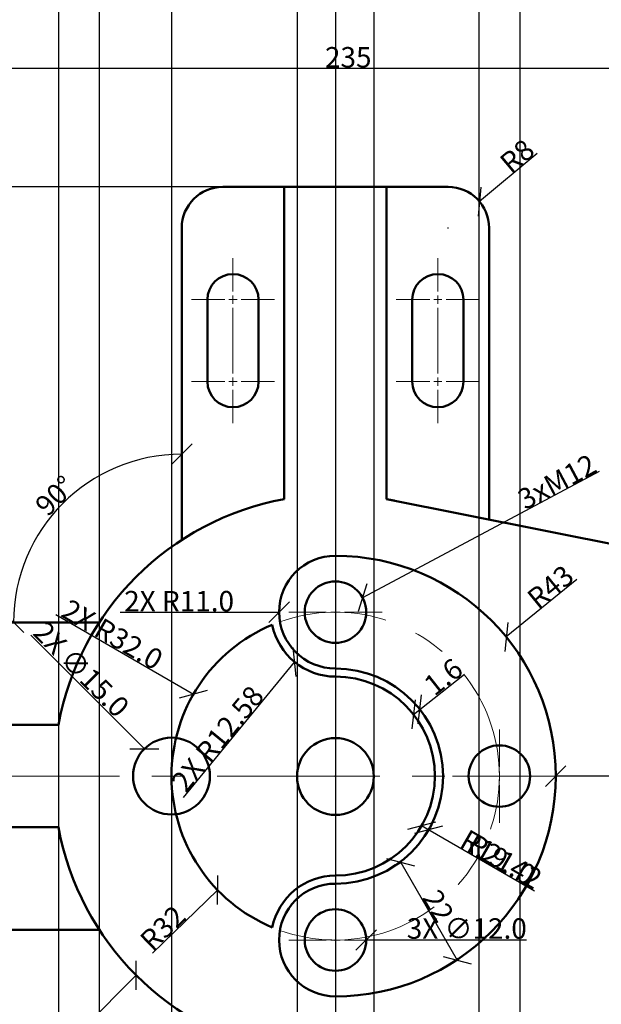
# Model space of a CAD drawing. Units: millimetres. Extents: x 263 to 611, y 50 to 522.
# Tile 3 of 5: x 364 to 478, y 157 to 349. Entities that reach past the tile are written whole.
import ezdxf

# ---------------------------------------------------------------- set-up
doc = ezdxf.new("R2010")
doc.units = ezdxf.units.MM
doc.header["$MEASUREMENT"] = 0
doc.linetypes.add('CENTER', pattern=[50.8, 31.75, -6.35, 6.35, -6.35])
for name, color, linetype, lineweight in [('M-CNTR', 1, 'CENTER', 18), ('M-DIMS', 2, 'Continuous', 25), ('M-OUTL', 7, 'Continuous', 50)]:
    doc.layers.add(name, color=color, linetype=linetype, lineweight=lineweight)
doc.styles.get("Standard").update_dxf_attribs({"font": 'arial.ttf'})
doc.dimstyles.get("Standard").update_dxf_attribs({"dimtxt": 4, "dimasz": 4, "dimexe": 0.18, "dimexo": 0.0625, "dimgap": 0.09, "dimtad": 1, "dimdec": 0, "dimzin": 0, "dimdsep": 46, "dimtxsty": 'Standard', "dimblk": 'OBLIQUE', "dimcen": 0.09, "dimclre": 251, "dimadec": 0, "dimazin": 0, "dimtfac": 1, "dimtdec": 0, "dimtofl": 0, "dimtmove": 0, "dimatfit": 3, "dimfxl": 1, "dimtolj": 1, "dimtzin": 0, "dimarcsym": 0})

# ---------------------------------------------------------------- blocks, each defined once
blk = doc.blocks.new('*U2')
at = {"layer": 'M-CNTR', "color": 0, "transparency": 16777216}
for p, q in [((0, 1.8), (0, 9.12)), ((-9.12, 0), (-1.8, 0)), ((1.8, 0), (9.12, 0)), ((0, -9.12), (0, -1.8))]:
    blk.add_line(p, q, dxfattribs=at)
at = {"layer": 'M-CNTR', "color": 0, "linetype": 'Continuous', "transparency": 16777216}
for p, q in [((-0.9, 0), (0.9, 0)), ((0, -0.9), (0, 0.9))]:
    blk.add_line(p, q, dxfattribs=at)
blk = doc.blocks.new('*U3')
at = {"layer": 'M-CNTR', "color": 0, "transparency": 16777216}
for p, q in [((0, 1.8), (0, 9.12)), ((-9.12, 0), (-1.8, 0)), ((1.8, 0), (9.12, 0)), ((0, -9.12), (0, -1.8))]:
    blk.add_line(p, q, dxfattribs=at)
at = {"layer": 'M-CNTR', "color": 0, "linetype": 'Continuous', "transparency": 16777216}
for p, q in [((-0.9, 0), (0.9, 0)), ((0, -0.9), (0, 0.9))]:
    blk.add_line(p, q, dxfattribs=at)
blk = doc.blocks.new('*U4')
at = {"layer": 'M-CNTR', "color": 0, "transparency": 16777216}
for p, q in [((0, 1.8), (0, 9.12)), ((-9.12, 0), (-1.8, 0)), ((1.8, 0), (9.12, 0)), ((0, -9.12), (0, -1.8))]:
    blk.add_line(p, q, dxfattribs=at)
at = {"layer": 'M-CNTR', "color": 0, "linetype": 'Continuous', "transparency": 16777216}
for p, q in [((-0.9, 0), (0.9, 0)), ((0, -0.9), (0, 0.9))]:
    blk.add_line(p, q, dxfattribs=at)
blk = doc.blocks.new('*U14')
at = {"layer": 'M-CNTR', "color": 0, "transparency": 16777216}
for p, q in [((0, 1.6), (0, 8.12)), ((-8.12, 0), (-1.6, 0)), ((1.6, 0), (8.12, 0)), ((0, -8.12), (0, -1.6))]:
    blk.add_line(p, q, dxfattribs=at)
at = {"layer": 'M-CNTR', "color": 0, "linetype": 'Continuous', "transparency": 16777216}
for p, q in [((-0.8, 0), (0.8, 0)), ((0, -0.8), (0, 0.8))]:
    blk.add_line(p, q, dxfattribs=at)
blk = doc.blocks.new('*U15')
at = {"layer": 'M-CNTR', "color": 0, "transparency": 16777216}
for p, q in [((0, 1.6), (0, 8.12)), ((-8.12, 0), (-1.6, 0)), ((1.6, 0), (8.12, 0)), ((0, -8.12), (0, -1.6))]:
    blk.add_line(p, q, dxfattribs=at)
at = {"layer": 'M-CNTR', "color": 0, "linetype": 'Continuous', "transparency": 16777216}
for p, q in [((-0.8, 0), (0.8, 0)), ((0, -0.8), (0, 0.8))]:
    blk.add_line(p, q, dxfattribs=at)
blk = doc.blocks.new('*U16')
at = {"layer": 'M-CNTR', "color": 0, "transparency": 16777216}
for p, q in [((0, 1.6), (0, 8.12)), ((-8.12, 0), (-1.6, 0)), ((1.6, 0), (8.12, 0)), ((0, -8.12), (0, -1.6))]:
    blk.add_line(p, q, dxfattribs=at)
at = {"layer": 'M-CNTR', "color": 0, "linetype": 'Continuous', "transparency": 16777216}
for p, q in [((-0.8, 0), (0.8, 0)), ((0, -0.8), (0, 0.8))]:
    blk.add_line(p, q, dxfattribs=at)
blk = doc.blocks.new('*U17')
at = {"layer": 'M-CNTR', "color": 0, "transparency": 16777216}
for p, q in [((0, 1.6), (0, 8.12)), ((-8.12, 0), (-1.6, 0)), ((1.6, 0), (8.12, 0)), ((0, -8.12), (0, -1.6))]:
    blk.add_line(p, q, dxfattribs=at)
at = {"layer": 'M-CNTR', "color": 0, "linetype": 'Continuous', "transparency": 16777216}
for p, q in [((-0.8, 0), (0.8, 0)), ((0, -0.8), (0, 0.8))]:
    blk.add_line(p, q, dxfattribs=at)
blk = doc.blocks.new('_Oblique')
at = {"color": 0, "linetype": 'ByBlock', "lineweight": -2}
blk.add_line((-0.5, -0.5), (0.5, 0.5), dxfattribs=at)
blk = doc.blocks.new('*D18')
at = {"layer": 'Defpoints', "color": 0, "transparency": 16777216}
for p in [(546.1, 339.25), (546.1, 231.08), (311.1, 223.08)]:
    blk.add_point(p, dxfattribs=at)
at = {"layer": 'M-DIMS', "color": 0, "lineweight": -2, "transparency": 16777216}
for p, q in [((311.1, 223.14), (311.1, 339.43)), ((311.1, 339.25), (546.1, 339.25)), ((546.1, 231.14), (546.1, 339.43))]:
    blk.add_line(p, q, dxfattribs=at)
at = {"layer": 'M-DIMS', "color": 0, "lineweight": -2, "transparency": 16777216, "xscale": 4, "yscale": 4, "zscale": 4, "rotation": 180}
blk.add_blockref('_Oblique', (311.1, 339.25), dxfattribs=at)
at = {"layer": 'M-DIMS', "color": 0, "lineweight": -2, "transparency": 16777216, "xscale": 4, "yscale": 4, "zscale": 4}
blk.add_blockref('_Oblique', (546.1, 339.25), dxfattribs=at)
at = {"layer": 'M-DIMS', "color": 0, "transparency": 16777216, "insert": (428.6, 341.39), "char_height": 4, "attachment_point": 5}
blk.add_mtext('\\A1;235', dxfattribs=at)
blk = doc.blocks.new('*D21')
at = {"layer": 'Defpoints', "color": 0, "transparency": 16777216}
for p in [(282.64, 316.08), (404.1, 316.08), (319.1, 231.08)]:
    blk.add_point(p, dxfattribs=at)
at = {"layer": 'M-DIMS', "color": 0, "lineweight": -2, "transparency": 16777216}
for p, q in [((404.04, 316.08), (282.46, 316.08)), ((282.64, 231.08), (282.64, 316.08)), ((319.04, 231.08), (282.46, 231.08))]:
    blk.add_line(p, q, dxfattribs=at)
at = {"layer": 'M-DIMS', "color": 0, "lineweight": -2, "transparency": 16777216, "xscale": 4, "yscale": 4, "zscale": 4}
for p, rotation in [((282.64, 316.08), 90), ((282.64, 231.08), 270)]:
    blk.add_blockref('_Oblique', p, dxfattribs=dict(at, rotation=rotation))
at = {"layer": 'M-DIMS', "color": 0, "transparency": 16777216, "insert": (280.51, 273.58), "char_height": 4, "attachment_point": 5, "rotation": 90}
blk.add_mtext('\\A1;85', dxfattribs=at)
blk = doc.blocks.new('*D22')
at = {"layer": 'Defpoints', "color": 0, "transparency": 16777216}
for p in [(404.1, 316.08), (267.8, 86.08), (404.1, 86.08)]:
    blk.add_point(p, dxfattribs=at)
at = {"layer": 'M-DIMS', "color": 0, "lineweight": -2, "transparency": 16777216}
for p, q in [((404.04, 316.08), (267.62, 316.08)), ((267.8, 316.08), (267.8, 86.08)), ((404.04, 86.08), (267.62, 86.08))]:
    blk.add_line(p, q, dxfattribs=at)
at = {"layer": 'M-DIMS', "color": 0, "lineweight": -2, "transparency": 16777216, "xscale": 4, "yscale": 4, "zscale": 4}
for p, rotation in [((267.8, 316.08), 90), ((267.8, 86.08), 270)]:
    blk.add_blockref('_Oblique', p, dxfattribs=dict(at, rotation=rotation))
at = {"layer": 'M-DIMS', "color": 0, "transparency": 16777216, "insert": (265.67, 201.08), "char_height": 4, "attachment_point": 5, "rotation": 90}
blk.add_mtext('\\A1;230', dxfattribs=at)
blk = doc.blocks.new('*D25')
at = {"layer": 'Defpoints', "color": 0, "transparency": 16777216}
for p in [(311.1, 201.08), (426.1, 201.08), (426.1, 140.57)]:
    blk.add_point(p, dxfattribs=at)
at = {"layer": 'M-DIMS', "color": 0, "lineweight": -2, "transparency": 16777216}
for p, q in [((311.1, 201.02), (311.1, 140.39)), ((426.1, 201.02), (426.1, 140.39)), ((311.1, 140.57), (426.1, 140.57))]:
    blk.add_line(p, q, dxfattribs=at)
at = {"layer": 'M-DIMS', "color": 0, "lineweight": -2, "transparency": 16777216, "xscale": 4, "yscale": 4, "zscale": 4, "rotation": 180}
blk.add_blockref('_Oblique', (311.1, 140.57), dxfattribs=at)
at = {"layer": 'M-DIMS', "color": 0, "lineweight": -2, "transparency": 16777216, "xscale": 4, "yscale": 4, "zscale": 4}
blk.add_blockref('_Oblique', (426.1, 140.57), dxfattribs=at)
at = {"layer": 'M-DIMS', "color": 0, "transparency": 16777216, "insert": (368.6, 142.7), "char_height": 4, "attachment_point": 5}
blk.add_mtext('\\A1;115', dxfattribs=at)
blk = doc.blocks.new('*D26')
at = {"layer": 'Defpoints', "color": 0, "transparency": 16777216}
for p in [(436.59, 182.89), (447.58, 163.83), (449.87, 165.15)]:
    blk.add_point(p, dxfattribs=at)
at = {"layer": 'M-DIMS', "color": 0, "lineweight": -2, "transparency": 16777216}
for p, q in [((436.64, 182.92), (439.04, 184.3)), ((438.88, 184.21), (449.87, 165.15)), ((447.64, 163.86), (450.03, 165.24))]:
    blk.add_line(p, q, dxfattribs=at)
at = {"layer": 'M-DIMS', "color": 0, "lineweight": -2, "transparency": 16777216, "xscale": 4, "yscale": 4, "zscale": 4}
for p, rotation in [((438.88, 184.21), 119.9728507659306), ((449.87, 165.15), 299.9728507659306)]:
    blk.add_blockref('_Oblique', p, dxfattribs=dict(at, rotation=rotation))
at = {"layer": 'M-DIMS', "color": 0, "transparency": 16777216, "insert": (446.19, 175.73), "char_height": 4, "attachment_point": 5, "rotation": 299.9729}
blk.add_mtext('\\A1;22', dxfattribs=at)
blk = doc.blocks.new('*D29')
at = {"layer": 'Defpoints', "color": 0, "transparency": 16777216}
for p in [(396.1, 308.08), (379.68, 259.52), (396.1, 247.18), (319.1, 231.08), (380, 231.08)]:
    blk.add_point(p, dxfattribs=at)
at = {"layer": 'M-DIMS', "color": 0, "lineweight": -2, "transparency": 16777216}
blk.add_arc((396.1, 231.08), 32.84, 90, 180, dxfattribs=at)
at = {"layer": 'M-DIMS', "color": 0, "lineweight": -2, "transparency": 16777216, "xscale": 4, "yscale": 4, "zscale": 4}
for p, rotation in [((396.1, 263.92), 359.9999999999999), ((363.26, 231.08), 269.9999999999999)]:
    blk.add_blockref('_Oblique', p, dxfattribs=dict(at, rotation=rotation))
at = {"layer": 'M-DIMS', "color": 0, "transparency": 16777216, "insert": (371.37, 255.81), "char_height": 4, "attachment_point": 5, "rotation": 45}
blk.add_mtext('\\A1;90°', dxfattribs=at)
blk = doc.blocks.new('*D30')
at = {"layer": 'Defpoints', "color": 0, "transparency": 16777216}
for p in [(454.24, 313.21), (448.1, 308.08)]:
    blk.add_point(p, dxfattribs=at)
at = {"layer": 'M-DIMS', "color": 0, "lineweight": -2, "transparency": 16777216}
for p, q in [((465.48, 322.59), (454.24, 313.21)), ((448.01, 308.08), (448.19, 308.08)), ((448.1, 307.99), (448.1, 308.17))]:
    blk.add_line(p, q, dxfattribs=at)
at = {"layer": 'M-DIMS', "color": 0, "lineweight": -2, "transparency": 16777216, "xscale": 4, "yscale": 4, "zscale": 4, "rotation": 219.8589270898177}
blk.add_blockref('_Oblique', (454.24, 313.21), dxfattribs=at)
at = {"layer": 'M-DIMS', "color": 0, "transparency": 16777216, "insert": (461.56, 322.1), "char_height": 4, "attachment_point": 5, "rotation": 39.8589}
blk.add_mtext('\\A1;R8', dxfattribs=at)
blk = doc.blocks.new('*D31')
at = {"layer": 'Defpoints', "color": 0, "transparency": 16777216}
for p in [(459.44, 228.24), (426.1, 201.08)]:
    blk.add_point(p, dxfattribs=at)
at = {"layer": 'M-DIMS', "color": 0, "lineweight": -2, "transparency": 16777216}
for p, q in [((473.19, 239.44), (459.44, 228.24)), ((426.01, 201.08), (426.19, 201.08)), ((426.1, 200.99), (426.1, 201.17))]:
    blk.add_line(p, q, dxfattribs=at)
at = {"layer": 'M-DIMS', "color": 0, "lineweight": -2, "transparency": 16777216, "xscale": 4, "yscale": 4, "zscale": 4, "rotation": 219.1694218645044}
blk.add_blockref('_Oblique', (459.44, 228.24), dxfattribs=at)
at = {"layer": 'M-DIMS', "color": 0, "transparency": 16777216, "insert": (468.07, 238.02), "char_height": 4, "attachment_point": 5, "rotation": 39.1694}
blk.add_mtext('\\A1;R43', dxfattribs=at)
blk = doc.blocks.new('*D32')
at = {"layer": 'Defpoints', "color": 0, "transparency": 16777216}
for p in [(426.1, 201.08), (403.1, 178.83)]:
    blk.add_point(p, dxfattribs=at)
at = {"layer": 'M-DIMS', "color": 0, "lineweight": -2, "transparency": 16777216}
for p, q in [((426.01, 201.08), (426.19, 201.08)), ((426.1, 200.99), (426.1, 201.17)), ((390.38, 166.52), (403.1, 178.83))]:
    blk.add_line(p, q, dxfattribs=at)
at = {"layer": 'M-DIMS', "color": 0, "lineweight": -2, "transparency": 16777216, "xscale": 4, "yscale": 4, "zscale": 4, "rotation": 44.055010952388}
blk.add_blockref('_Oblique', (403.1, 178.83), dxfattribs=at)
at = {"layer": 'M-DIMS', "color": 0, "transparency": 16777216, "insert": (392.38, 171.43), "char_height": 4, "attachment_point": 5, "rotation": 44.055}
blk.add_mtext('\\A1;R32', dxfattribs=at)
blk = doc.blocks.new('*D33')
at = {"layer": 'Defpoints', "color": 0, "transparency": 16777216}
for p in [(442.57, 214.11), (442.57, 214.11), (441.33, 213.13)]:
    blk.add_point(p, dxfattribs=at)
at = {"layer": 'M-DIMS', "color": 0, "lineweight": -2, "transparency": 16777216}
for p, q in [((442.57, 214.11), (451.26, 220.98)), ((441.33, 213.13), (442.57, 214.11)), ((442.61, 214.06), (442.68, 213.97)), ((441.37, 213.08), (441.44, 212.99))]:
    blk.add_line(p, q, dxfattribs=at)
at = {"layer": 'M-DIMS', "color": 0, "lineweight": -2, "transparency": 16777216, "xscale": 4, "yscale": 4, "zscale": 4}
for p, rotation in [((441.33, 213.13), 218.3421878076332), ((442.57, 214.11), 38.34218780763318)]:
    blk.add_blockref('_Oblique', p, dxfattribs=dict(at, rotation=rotation))
at = {"layer": 'M-DIMS', "color": 0, "transparency": 16777216, "insert": (447.16, 220.46), "char_height": 4, "attachment_point": 5, "rotation": 38.3422}
blk.add_mtext('\\A1;1.6', dxfattribs=at)
blk = doc.blocks.new('*D35')
at = {"layer": 'Defpoints', "color": 0, "transparency": 16777216}
for p in [(431.39, 235.9), (420.8, 230.26)]:
    blk.add_point(p, dxfattribs=at)
at = {"layer": 'M-DIMS', "color": 0, "lineweight": -2, "transparency": 16777216}
for p, q in [((477.59, 260.53), (431.39, 235.9)), ((426.01, 233.08), (426.19, 233.08)), ((426.1, 232.99), (426.1, 233.17))]:
    blk.add_line(p, q, dxfattribs=at)
at = {"layer": 'M-DIMS', "color": 0, "lineweight": -2, "transparency": 16777216, "xscale": 4, "yscale": 4, "zscale": 4, "rotation": 208.0625642859589}
blk.add_blockref('_Oblique', (431.39, 235.9), dxfattribs=at)
at = {"layer": 'M-DIMS', "color": 0, "transparency": 16777216, "insert": (469.34, 258.55), "char_height": 4, "attachment_point": 5, "rotation": 28.0626}
blk.add_mtext('\\A1;3xM12', dxfattribs=at)
blk = doc.blocks.new('SLOT-10x26')
for p, q in [((0, 5), (0, 21)), ((10, 5), (10, 21))]:
    blk.add_line(p, q)
for centre, start, end in [((5, 21), 0, 180), ((5, 5), 180, 0)]:
    blk.add_arc(centre, 5, start, end)
blk = doc.blocks.new('*D53')
at = {"layer": 'Defpoints', "color": 0, "transparency": 16777216}
for p in [(578.1, 423.27), (311.1, 383.27), (578.1, 52.26)]:
    blk.add_point(p, dxfattribs=at)
at = {"layer": 'M-DIMS', "color": 251, "lineweight": -2, "transparency": 16777216}
for p, q in [((578.1, 423.21), (578.1, 52.08)), ((311.1, 383.21), (311.1, 52.08))]:
    blk.add_line(p, q, dxfattribs=at)
at = {"layer": 'M-DIMS', "color": 0, "lineweight": -2, "transparency": 16777216}
blk.add_line((311.1, 52.26), (578.1, 52.26), dxfattribs=at)
at = {"layer": 'M-DIMS', "color": 0, "lineweight": -2, "transparency": 16777216, "xscale": 4, "yscale": 4, "zscale": 4, "rotation": 180}
blk.add_blockref('_Oblique', (311.1, 52.26), dxfattribs=at)
at = {"layer": 'M-DIMS', "color": 0, "lineweight": -2, "transparency": 16777216, "xscale": 4, "yscale": 4, "zscale": 4}
blk.add_blockref('_Oblique', (578.1, 52.26), dxfattribs=at)
at = {"layer": 'M-DIMS', "color": 0, "transparency": 16777216, "insert": (444.6, 54.39), "char_height": 4, "attachment_point": 5}
blk.add_mtext('\\A1;267.0', dxfattribs=at)
blk = doc.blocks.new('*D56')
at = {"layer": 'Defpoints', "color": 0, "transparency": 16777216}
for p in [(454.1, 410.27), (462.1, 410.27), (462.1, 52.26)]:
    blk.add_point(p, dxfattribs=at)
at = {"layer": 'M-DIMS', "color": 251, "lineweight": -2, "transparency": 16777216}
for p, q in [((454.1, 410.21), (454.1, 52.08)), ((462.1, 410.21), (462.1, 52.08))]:
    blk.add_line(p, q, dxfattribs=at)
at = {"layer": 'M-DIMS', "color": 0, "lineweight": -2, "transparency": 16777216}
blk.add_line((454.1, 52.26), (462.1, 52.26), dxfattribs=at)
at = {"layer": 'M-DIMS', "color": 0, "lineweight": -2, "transparency": 16777216, "xscale": 4, "yscale": 4, "zscale": 4, "rotation": 180}
blk.add_blockref('_Oblique', (454.1, 52.26), dxfattribs=at)
at = {"layer": 'M-DIMS', "color": 0, "lineweight": -2, "transparency": 16777216, "xscale": 4, "yscale": 4, "zscale": 4}
blk.add_blockref('_Oblique', (462.1, 52.26), dxfattribs=at)
at = {"layer": 'M-DIMS', "color": 0, "transparency": 16777216, "insert": (458.1, 54.39), "char_height": 4, "attachment_point": 5}
blk.add_mtext('\\A1;8.0', dxfattribs=at)
blk = doc.blocks.new('*D57')
at = {"layer": 'Defpoints', "color": 0, "transparency": 16777216}
for p in [(372.02, 403.27), (311.1, 383.27), (372.02, 52.26)]:
    blk.add_point(p, dxfattribs=at)
at = {"layer": 'M-DIMS', "color": 251, "lineweight": -2, "transparency": 16777216}
for p, q in [((372.02, 403.21), (372.02, 52.08)), ((311.1, 383.21), (311.1, 52.08))]:
    blk.add_line(p, q, dxfattribs=at)
at = {"layer": 'M-DIMS', "color": 0, "lineweight": -2, "transparency": 16777216}
blk.add_line((311.1, 52.26), (372.02, 52.26), dxfattribs=at)
at = {"layer": 'M-DIMS', "color": 0, "lineweight": -2, "transparency": 16777216, "xscale": 4, "yscale": 4, "zscale": 4, "rotation": 180}
blk.add_blockref('_Oblique', (311.1, 52.26), dxfattribs=at)
at = {"layer": 'M-DIMS', "color": 0, "lineweight": -2, "transparency": 16777216, "xscale": 4, "yscale": 4, "zscale": 4}
blk.add_blockref('_Oblique', (372.02, 52.26), dxfattribs=at)
at = {"layer": 'M-DIMS', "color": 0, "transparency": 16777216, "insert": (341.56, 54.39), "char_height": 4, "attachment_point": 5}
blk.add_mtext('\\A1;60.92', dxfattribs=at)
blk = doc.blocks.new('*D58')
at = {"layer": 'Defpoints', "color": 0, "transparency": 16777216}
for p in [(372.02, 403.27), (380, 383.27), (380, 52.26)]:
    blk.add_point(p, dxfattribs=at)
at = {"layer": 'M-DIMS', "color": 251, "lineweight": -2, "transparency": 16777216}
for p, q in [((372.02, 403.21), (372.02, 52.08)), ((380, 383.21), (380, 52.08))]:
    blk.add_line(p, q, dxfattribs=at)
at = {"layer": 'M-DIMS', "color": 0, "lineweight": -2, "transparency": 16777216}
for p, q in [((372.02, 52.26), (380, 52.26)), ((380, 52.26), (397.64, 52.26))]:
    blk.add_line(p, q, dxfattribs=at)
at = {"layer": 'M-DIMS', "color": 0, "lineweight": -2, "transparency": 16777216, "xscale": 4, "yscale": 4, "zscale": 4, "rotation": 180}
blk.add_blockref('_Oblique', (372.02, 52.26), dxfattribs=at)
at = {"layer": 'M-DIMS', "color": 0, "lineweight": -2, "transparency": 16777216, "xscale": 4, "yscale": 4, "zscale": 4}
blk.add_blockref('_Oblique', (380, 52.26), dxfattribs=at)
at = {"layer": 'M-DIMS', "color": 0, "transparency": 16777216, "insert": (390.82, 54.39), "char_height": 4, "attachment_point": 5}
blk.add_mtext('\\A1;7.986', dxfattribs=at)
blk = doc.blocks.new('*D59')
at = {"layer": 'Defpoints', "color": 0, "transparency": 16777216}
for p in [(380, 383.27), (394.1, 383.27), (394.1, 52.26)]:
    blk.add_point(p, dxfattribs=at)
at = {"layer": 'M-DIMS', "color": 251, "lineweight": -2, "transparency": 16777216}
for p, q in [((380, 383.21), (380, 52.08)), ((394.1, 383.21), (394.1, 52.08))]:
    blk.add_line(p, q, dxfattribs=at)
at = {"layer": 'M-DIMS', "color": 0, "lineweight": -2, "transparency": 16777216}
for p, q in [((380, 52.26), (394.1, 52.26)), ((394.1, 52.26), (414.52, 52.26))]:
    blk.add_line(p, q, dxfattribs=at)
at = {"layer": 'M-DIMS', "color": 0, "lineweight": -2, "transparency": 16777216, "xscale": 4, "yscale": 4, "zscale": 4, "rotation": 180}
blk.add_blockref('_Oblique', (380, 52.26), dxfattribs=at)
at = {"layer": 'M-DIMS', "color": 0, "lineweight": -2, "transparency": 16777216, "xscale": 4, "yscale": 4, "zscale": 4}
blk.add_blockref('_Oblique', (394.1, 52.26), dxfattribs=at)
at = {"layer": 'M-DIMS', "color": 0, "transparency": 16777216, "insert": (406.31, 54.39), "char_height": 4, "attachment_point": 5}
blk.add_mtext('\\A1;14.098', dxfattribs=at)
blk = doc.blocks.new('*D60')
at = {"layer": 'Defpoints', "color": 0, "transparency": 16777216}
for p in [(418.6, 403.27), (394.1, 383.27), (418.6, 52.26)]:
    blk.add_point(p, dxfattribs=at)
at = {"layer": 'M-DIMS', "color": 251, "lineweight": -2, "transparency": 16777216}
for p, q in [((418.6, 403.21), (418.6, 52.08)), ((394.1, 383.21), (394.1, 52.08))]:
    blk.add_line(p, q, dxfattribs=at)
at = {"layer": 'M-DIMS', "color": 0, "lineweight": -2, "transparency": 16777216}
blk.add_line((394.1, 52.26), (418.6, 52.26), dxfattribs=at)
at = {"layer": 'M-DIMS', "color": 0, "lineweight": -2, "transparency": 16777216, "xscale": 4, "yscale": 4, "zscale": 4, "rotation": 180}
blk.add_blockref('_Oblique', (394.1, 52.26), dxfattribs=at)
at = {"layer": 'M-DIMS', "color": 0, "lineweight": -2, "transparency": 16777216, "xscale": 4, "yscale": 4, "zscale": 4}
blk.add_blockref('_Oblique', (418.6, 52.26), dxfattribs=at)
at = {"layer": 'M-DIMS', "color": 0, "transparency": 16777216, "insert": (406.35, 54.39), "char_height": 4, "attachment_point": 5}
blk.add_mtext('\\A1;24.5', dxfattribs=at)
blk = doc.blocks.new('*D61')
at = {"layer": 'Defpoints', "color": 0, "transparency": 16777216}
for p in [(418.6, 403.27), (426.1, 378.63), (426.1, 52.26)]:
    blk.add_point(p, dxfattribs=at)
at = {"layer": 'M-DIMS', "color": 251, "lineweight": -2, "transparency": 16777216}
for p, q in [((418.6, 403.21), (418.6, 52.08)), ((426.1, 378.57), (426.1, 52.08))]:
    blk.add_line(p, q, dxfattribs=at)
at = {"layer": 'M-DIMS', "color": 0, "lineweight": -2, "transparency": 16777216}
blk.add_line((418.6, 52.26), (426.1, 52.26), dxfattribs=at)
at = {"layer": 'M-DIMS', "color": 0, "lineweight": -2, "transparency": 16777216, "xscale": 4, "yscale": 4, "zscale": 4, "rotation": 180}
blk.add_blockref('_Oblique', (418.6, 52.26), dxfattribs=at)
at = {"layer": 'M-DIMS', "color": 0, "lineweight": -2, "transparency": 16777216, "xscale": 4, "yscale": 4, "zscale": 4}
blk.add_blockref('_Oblique', (426.1, 52.26), dxfattribs=at)
at = {"layer": 'M-DIMS', "color": 0, "transparency": 16777216, "insert": (422.35, 54.38), "char_height": 4, "attachment_point": 5}
blk.add_mtext('\\A1;7.5', dxfattribs=at)
blk = doc.blocks.new('*D62')
at = {"layer": 'Defpoints', "color": 0, "transparency": 16777216}
for p in [(433.6, 383.27), (426.1, 378.63), (433.6, 52.26)]:
    blk.add_point(p, dxfattribs=at)
at = {"layer": 'M-DIMS', "color": 251, "lineweight": -2, "transparency": 16777216}
for p, q in [((433.6, 383.21), (433.6, 52.08)), ((426.1, 378.57), (426.1, 52.08))]:
    blk.add_line(p, q, dxfattribs=at)
at = {"layer": 'M-DIMS', "color": 0, "lineweight": -2, "transparency": 16777216}
blk.add_line((426.1, 52.26), (433.6, 52.26), dxfattribs=at)
at = {"layer": 'M-DIMS', "color": 0, "lineweight": -2, "transparency": 16777216, "xscale": 4, "yscale": 4, "zscale": 4, "rotation": 180}
blk.add_blockref('_Oblique', (426.1, 52.26), dxfattribs=at)
at = {"layer": 'M-DIMS', "color": 0, "lineweight": -2, "transparency": 16777216, "xscale": 4, "yscale": 4, "zscale": 4}
blk.add_blockref('_Oblique', (433.6, 52.26), dxfattribs=at)
at = {"layer": 'M-DIMS', "color": 0, "transparency": 16777216, "insert": (429.85, 54.38), "char_height": 4, "attachment_point": 5}
blk.add_mtext('\\A1;7.5', dxfattribs=at)
blk = doc.blocks.new('*D69')
at = {"layer": 'Defpoints', "color": 0, "transparency": 16777216}
for p in [(426.1, 201.08), (387.21, 162.19)]:
    blk.add_point(p, dxfattribs=at)
at = {"layer": 'M-DIMS', "color": 251, "lineweight": -2, "transparency": 16777216}
for p, q in [((426.01, 201.08), (426.19, 201.08)), ((426.1, 200.99), (426.1, 201.17))]:
    blk.add_line(p, q, dxfattribs=at)
at = {"layer": 'M-DIMS', "color": 0, "lineweight": -2, "transparency": 16777216}
blk.add_line((355.69, 130.68), (387.21, 162.19), dxfattribs=at)
at = {"layer": 'M-DIMS', "color": 0, "lineweight": -2, "transparency": 16777216, "xscale": 4, "yscale": 4, "zscale": 4, "rotation": 44.99977533015295}
blk.add_blockref('_Oblique', (387.21, 162.19), dxfattribs=at)
at = {"layer": 'M-DIMS', "color": 0, "transparency": 16777216, "insert": (362.37, 140.36), "char_height": 4, "attachment_point": 5, "rotation": 44.9998}
blk.add_mtext('\\A1;4X R55.0', dxfattribs=at)
blk = doc.blocks.new('*D70')
at = {"layer": 'Defpoints', "color": 0, "transparency": 16777216}
for p in [(426.1, 201.08), (469.1, 201.08)]:
    blk.add_point(p, dxfattribs=at)
at = {"layer": 'M-DIMS', "color": 251, "lineweight": -2, "transparency": 16777216}
for p, q in [((426.01, 201.08), (426.19, 201.08)), ((426.1, 200.99), (426.1, 201.17))]:
    blk.add_line(p, q, dxfattribs=at)
at = {"layer": 'M-DIMS', "color": 0, "lineweight": -2, "transparency": 16777216}
blk.add_line((502.09, 201.08), (469.1, 201.08), dxfattribs=at)
at = {"layer": 'M-DIMS', "color": 0, "lineweight": -2, "transparency": 16777216, "xscale": 4, "yscale": 4, "zscale": 4, "rotation": 180.0006262561947}
blk.add_blockref('_Oblique', (469.1, 201.08), dxfattribs=at)
at = {"layer": 'M-DIMS', "color": 0, "transparency": 16777216, "insert": (494.9, 203.22), "char_height": 4, "attachment_point": 5, "rotation": 0.0006}
blk.add_mtext('\\A1;R43.0', dxfattribs=at)
blk = doc.blocks.new('*D71')
at = {"layer": 'Defpoints', "color": 0, "transparency": 16777216}
for p in [(398.4, 217.1), (426.1, 201.08)]:
    blk.add_point(p, dxfattribs=at)
at = {"layer": 'M-DIMS', "color": 0, "lineweight": -2, "transparency": 16777216}
blk.add_line((371.52, 232.64), (398.4, 217.1), dxfattribs=at)
at = {"layer": 'M-DIMS', "color": 251, "lineweight": -2, "transparency": 16777216}
for p, q in [((426.01, 201.08), (426.19, 201.08)), ((426.1, 200.99), (426.1, 201.17))]:
    blk.add_line(p, q, dxfattribs=at)
at = {"layer": 'M-DIMS', "color": 0, "lineweight": -2, "transparency": 16777216, "xscale": 4, "yscale": 4, "zscale": 4, "rotation": 329.9588428914435}
blk.add_blockref('_Oblique', (398.4, 217.1), dxfattribs=at)
at = {"layer": 'M-DIMS', "color": 0, "transparency": 16777216, "insert": (382.56, 228.72), "char_height": 4, "attachment_point": 5, "rotation": 329.9588}
blk.add_mtext('\\A1;2X R32.0', dxfattribs=at)
blk = doc.blocks.new('*D74')
at = {"layer": 'Defpoints', "color": 0, "transparency": 16777216}
for p in [(426.1, 201.08), (442.92, 191.37)]:
    blk.add_point(p, dxfattribs=at)
at = {"layer": 'M-DIMS', "color": 251, "lineweight": -2, "transparency": 16777216}
for p, q in [((426.01, 201.08), (426.19, 201.08)), ((426.1, 200.99), (426.1, 201.17))]:
    blk.add_line(p, q, dxfattribs=at)
at = {"layer": 'M-DIMS', "color": 0, "lineweight": -2, "transparency": 16777216}
blk.add_line((464.97, 178.64), (442.92, 191.37), dxfattribs=at)
at = {"layer": 'M-DIMS', "color": 0, "lineweight": -2, "transparency": 16777216, "xscale": 4, "yscale": 4, "zscale": 4, "rotation": 150.0004448494699}
blk.add_blockref('_Oblique', (442.92, 191.37), dxfattribs=at)
at = {"layer": 'M-DIMS', "color": 0, "transparency": 16777216, "insert": (458.47, 184.85), "char_height": 4, "attachment_point": 5, "rotation": 330.0004}
blk.add_mtext('\\A1;R19.42', dxfattribs=at)
blk = doc.blocks.new('*D75')
at = {"layer": 'Defpoints', "color": 0, "transparency": 16777216}
for p in [(426.1, 201.08), (444.29, 190.58)]:
    blk.add_point(p, dxfattribs=at)
at = {"layer": 'M-DIMS', "color": 251, "lineweight": -2, "transparency": 16777216}
for p, q in [((426.01, 201.08), (426.19, 201.08)), ((426.1, 200.99), (426.1, 201.17))]:
    blk.add_line(p, q, dxfattribs=at)
at = {"layer": 'M-DIMS', "color": 0, "lineweight": -2, "transparency": 16777216}
blk.add_line((463.67, 179.39), (444.29, 190.58), dxfattribs=at)
at = {"layer": 'M-DIMS', "color": 0, "lineweight": -2, "transparency": 16777216, "xscale": 4, "yscale": 4, "zscale": 4, "rotation": 149.9986253737685}
blk.add_blockref('_Oblique', (444.29, 190.58), dxfattribs=at)
at = {"layer": 'M-DIMS', "color": 0, "transparency": 16777216, "insert": (458.51, 184.83), "char_height": 4, "attachment_point": 5, "rotation": 329.9986}
blk.add_mtext('\\A1;R21.0', dxfattribs=at)
blk = doc.blocks.new('*D76')
at = {"layer": 'Defpoints', "color": 0, "transparency": 16777216}
for p in [(426.1, 233.08), (418.13, 223.35)]:
    blk.add_point(p, dxfattribs=at)
at = {"layer": 'M-DIMS', "color": 251, "lineweight": -2, "transparency": 16777216}
for p, q in [((426.01, 233.08), (426.19, 233.08)), ((426.1, 232.99), (426.1, 233.17))]:
    blk.add_line(p, q, dxfattribs=at)
at = {"layer": 'M-DIMS', "color": 0, "lineweight": -2, "transparency": 16777216}
blk.add_line((396.46, 196.92), (418.13, 223.35), dxfattribs=at)
at = {"layer": 'M-DIMS', "color": 0, "lineweight": -2, "transparency": 16777216, "xscale": 4, "yscale": 4, "zscale": 4, "rotation": 50.66655948847605}
blk.add_blockref('_Oblique', (418.13, 223.35), dxfattribs=at)
at = {"layer": 'M-DIMS', "color": 0, "transparency": 16777216, "insert": (403.11, 208.39), "char_height": 4, "attachment_point": 5, "rotation": 50.6666}
blk.add_mtext('\\A1;2X R12.58', dxfattribs=at)
blk = doc.blocks.new('*D77')
at = {"layer": 'Defpoints', "color": 0, "transparency": 16777216}
for p in [(415.1, 233.08), (426.1, 233.08)]:
    blk.add_point(p, dxfattribs=at)
at = {"layer": 'M-DIMS', "color": 0, "lineweight": -2, "transparency": 16777216}
blk.add_line((384.05, 233.08), (415.1, 233.08), dxfattribs=at)
at = {"layer": 'M-DIMS', "color": 251, "lineweight": -2, "transparency": 16777216}
for p, q in [((426.01, 233.08), (426.19, 233.08)), ((426.1, 232.99), (426.1, 233.17))]:
    blk.add_line(p, q, dxfattribs=at)
at = {"layer": 'M-DIMS', "color": 0, "lineweight": -2, "transparency": 16777216, "xscale": 4, "yscale": 4, "zscale": 4, "rotation": 359.9975519076041}
blk.add_blockref('_Oblique', (415.1, 233.08), dxfattribs=at)
at = {"layer": 'M-DIMS', "color": 0, "transparency": 16777216, "insert": (395.58, 235.22), "char_height": 4, "attachment_point": 5, "rotation": 359.9976}
blk.add_mtext('\\A1;2X R11.0', dxfattribs=at)
blk = doc.blocks.new('*D78')
at = {"layer": 'Defpoints', "color": 0, "transparency": 16777216}
for p in [(420.1, 169.08), (432.1, 169.08)]:
    blk.add_point(p, dxfattribs=at)
at = {"layer": 'M-DIMS', "color": 251, "lineweight": -2, "transparency": 16777216}
for p, q in [((426.1, 168.99), (426.1, 169.17)), ((426.01, 169.08), (426.19, 169.08))]:
    blk.add_line(p, q, dxfattribs=at)
at = {"layer": 'M-DIMS', "color": 0, "lineweight": -2, "transparency": 16777216}
blk.add_line((463.39, 169.08), (432.1, 169.08), dxfattribs=at)
at = {"layer": 'M-DIMS', "color": 0, "lineweight": -2, "transparency": 16777216, "xscale": 4, "yscale": 4, "zscale": 4, "rotation": 180.0044881693859}
blk.add_blockref('_Oblique', (432.1, 169.08), dxfattribs=at)
at = {"layer": 'M-DIMS', "color": 0, "transparency": 16777216, "insert": (451.74, 171.33), "char_height": 4, "attachment_point": 5, "rotation": 0.0045}
blk.add_mtext('\\A1;3X ∅12.0', dxfattribs=at)
blk = doc.blocks.new('*D79')
at = {"layer": 'Defpoints', "color": 0, "transparency": 16777216}
for p in [(388.81, 206.39), (399.39, 195.77)]:
    blk.add_point(p, dxfattribs=at)
at = {"layer": 'M-DIMS', "color": 0, "lineweight": -2, "transparency": 16777216}
blk.add_line((366.67, 228.61), (388.81, 206.39), dxfattribs=at)
at = {"layer": 'M-DIMS', "color": 251, "lineweight": -2, "transparency": 16777216}
for p, q in [((394.01, 201.08), (394.19, 201.08)), ((394.1, 200.99), (394.1, 201.17))]:
    blk.add_line(p, q, dxfattribs=at)
at = {"layer": 'M-DIMS', "color": 0, "lineweight": -2, "transparency": 16777216, "xscale": 4, "yscale": 4, "zscale": 4, "rotation": 314.8940417265354}
blk.add_blockref('_Oblique', (388.81, 206.39), dxfattribs=at)
at = {"layer": 'M-DIMS', "color": 0, "transparency": 16777216, "insert": (376.51, 221.92), "char_height": 4, "attachment_point": 5, "rotation": 314.894}
blk.add_mtext('\\A1;2X ∅15.0', dxfattribs=at)

msp = doc.modelspace()

# ---------------------------------------------------------------- linework, layer by layer
at = {"layer": 'M-CNTR'}
for p, q in [((426.0988, 323.9478), (426.0988, 74.3557)), ((587.1329, 201.0815), (311.0988, 201.0815))]:
    msp.add_line(p, q, dxfattribs=at)
msp.add_arc((426.0988, 201.0815), 32, 250.206293, 109.793707, dxfattribs=at)
at = {"layer": 'M-OUTL'}
for p, q in [((404.0988, 316.0815), (448.0988, 316.0815)), ((416.0988, 316.0815), (416.0988, 255.1648)), ((436.0988, 316.0815), (436.0988, 255.1648)), ((396.0988, 308.0815), (396.0988, 247.1793)), ((456.0988, 308.0815), (456.0988, 251.1718)), ((552.2661, 231.9719), (436.0988, 255.1648)), ((319.0988, 231.0815), (380.0011, 231.0815)), ((311.0988, 211.0815), (372.0156, 211.0815)), ((311.0988, 191.0815), (372.0156, 191.0815)), ((319.0988, 171.0815), (380.0011, 171.0815))]:
    msp.add_line(p, q, dxfattribs=at)
for centre, radius in [((426.0988, 233.0815), 6), ((394.0988, 201.0815), 7.5), ((426.0988, 200.9915), 7.5), ((458.0988, 201.0815), 6), ((426.0988, 169.0815), 6)]:
    msp.add_circle(centre, radius, dxfattribs=at)
for centre, radius, start, end in [((404.0988, 308.0815), 8, 90, 180), ((448.0988, 308.0815), 8, 0, 90), ((426.0988, 201.0815), 55, 100.475682, 169.524318), ((426.0988, 201.0815), 55, 77.894283, 79.524318), ((426.0988, 233.0815), 11, 90, 270), ((426.0988, 201.0815), 43, 270, 90), ((426.0988, 201.0815), 32, 112.67203, 247.32797), ((426.0988, 233.0815), 12.58, 191.336015, 270), ((426.0988, 201.0815), 21, 270, 90), ((426.0988, 201.0815), 19.42, 270, 90), ((426.0988, 201.0815), 55, 190.475682, 259.524318), ((426.0988, 169.0815), 12.58, 90, 168.663985), ((426.0988, 169.0815), 11, 90, 270)]:
    msp.add_arc(centre, radius, start, end, dxfattribs=at)

# ---------------------------------------------------------------- block references
at = {"layer": 'M-CNTR'}
for name, p in [('*U16', (406.0988, 294.0815)), ('*U15', (446.0988, 294.0815)), ('*U17', (406.0988, 278.0815)), ('*U14', (446.0988, 278.0815)), ('*U2', (426.0988, 169.0815))]:
    msp.add_blockref(name, p, dxfattribs=at)
for name, p, rotation in [('*U4', (426.0988, 233.0815), 180), ('*U3', (458.0988, 201.0815), 90.00000000000003)]:
    msp.add_blockref(name, p, dxfattribs=dict(at, rotation=rotation))
at = {"layer": 'M-OUTL', "rotation": 180}
for p in [(411.0987, 299.0811), (451.0987, 299.0811)]:
    msp.add_blockref('SLOT-10x26', p, dxfattribs=at)

# ---------------------------------------------------------------- dimensions: what is measured, and where the dimension line sits
at = {"layer": 'M-DIMS'}
for base, p1, p2, override, picture, middle in [((578.0988, 52.2557), (311.0988, 383.2727), (578.0988, 423.2727), {"dimdec": 1, "dimlfac": 1, "dimrnd": 0, "dimzin": 0, "dimdsep": 46, "dimlunit": 2}, '*D53', (444.5988, 54.388)), ((462.0988, 52.2557), (454.0988, 410.2727), (462.0988, 410.2727), {"dimdec": 1, "dimlfac": 1, "dimrnd": 0, "dimzin": 0, "dimdsep": 46, "dimlunit": 2}, '*D56', (458.0988, 54.388)), ((372.0156, 52.2557), (311.0988, 383.2727), (372.0156, 403.2727), {"dimdec": 2, "dimlfac": 1, "dimrnd": 0, "dimzin": 0, "dimdsep": 46, "dimlunit": 2}, '*D57', (341.5572, 54.388)), ((380.00111, 52.25572), (372.01556, 403.2727), (380.00111, 383.2727), {"dimdec": 3, "dimlfac": 1, "dimrnd": 0, "dimzin": 0, "dimdsep": 46, "dimlunit": 2}, '*D58', (390.82235, 54.38801)), ((418.5988, 52.2557), (394.0988, 383.2727), (418.5988, 403.2727), {"dimdec": 1, "dimlfac": 1, "dimrnd": 0, "dimzin": 0, "dimdsep": 46, "dimlunit": 2}, '*D60', (406.3488, 54.388)), ((426.0988, 52.2557), (418.5988, 403.2727), (426.0988, 378.6323), {"dimdec": 1, "dimlfac": 1, "dimrnd": 0, "dimzin": 0, "dimdsep": 46, "dimlunit": 2}, '*D61', (422.3488, 54.3798)), ((394.0988, 52.2557), (380.0011, 383.2727), (394.0988, 383.2727), {"dimdec": 3, "dimlfac": 1, "dimrnd": 0, "dimzin": 0, "dimdsep": 46, "dimlunit": 2}, '*D59', (406.3075, 54.388)), ((433.5988, 52.2557), (426.0988, 378.6323), (433.5988, 383.2727), {"dimdec": 1, "dimlfac": 1, "dimrnd": 0, "dimzin": 0, "dimdsep": 46, "dimlunit": 2}, '*D62', (429.8488, 54.3798)), ((546.0988, 339.2528), (311.0988, 223.0815), (546.0988, 231.0815), {"dimclrd": 0, "dimclre": 0, "dimclrt": 0}, '*D18', (428.5988, 341.3864)), ((426.0988, 140.5664), (311.0988, 201.0815), (426.0988, 201.0815), {"dimclrd": 0, "dimclre": 0, "dimclrt": 0}, '*D25', (368.5988, 142.6987))]:
    dim = msp.add_linear_dim(base=base, p1=p1, p2=p2, dimstyle='Standard', override=override, dxfattribs=at)
    dim.commit()
    dim.dimension.update_dxf_attribs({"geometry": picture, "text_midpoint": middle})
for center, mpoint, override, picture, middle in [((448.0988, 308.0815), (454.2398, 313.2087), {"dimclrd": 0, "dimclre": 0, "dimclrt": 0}, '*D30', (461.5621, 322.1)), ((426.0988, 201.0815), (459.4359, 228.241), {"dimclrd": 0, "dimclre": 0, "dimclrt": 0}, '*D31', (468.0654, 238.0234)), ((426.0988, 201.0815), (403.1013, 178.8304), {"dimclrd": 0, "dimclre": 0, "dimclrt": 0}, '*D32', (392.3838, 171.4296)), ((426.0988, 201.0815), (442.9171, 191.3717), {"dimdec": 2, "dimlfac": 1, "dimrnd": 0, "dimzin": 0, "dimdsep": 46, "dimlunit": 2}, '*D74', (458.4741, 184.8521)), ((426.0988, 201.0815), (444.2851, 190.5811), {"dimdec": 1, "dimlfac": 1, "dimrnd": 0, "dimzin": 0, "dimdsep": 46, "dimlunit": 2}, '*D75', (458.5081, 184.8312))]:
    dim = msp.add_radius_dim(center=center, mpoint=mpoint, dimstyle='Standard', override=override, dxfattribs=at)
    dim.commit()
    dim.dimension.update_dxf_attribs({"geometry": picture, "text_midpoint": middle})
for base, p1, p2, picture, middle in [((267.7992, 86.0815), (404.0988, 316.0815), (404.0988, 86.0815), '*D22', (265.6656, 201.0815)), ((282.6439, 316.0815), (319.0988, 231.0815), (404.0988, 316.0815), '*D21', (280.5117, 273.5815))]:
    dim = msp.add_linear_dim(base=base, p1=p1, p2=p2, angle=90, dimstyle='Standard', override={"dimclrd": 0, "dimclre": 0, "dimclrt": 0}, dxfattribs=at)
    dim.commit()
    dim.dimension.update_dxf_attribs({"geometry": picture, "text_midpoint": middle})
dim = msp.add_angular_dim_2l(base=(379.6771, 259.5248), line1=((396.0988, 308.0815), (396.0988, 247.1793)), line2=((319.0988, 231.0815), (380.0011, 231.0815)), dimstyle='Standard', override={"dimclrd": 0, "dimclre": 0, "dimclrt": 0}, dxfattribs=at)
dim.commit()
dim.dimension.update_dxf_attribs({"geometry": '*D29', "text_midpoint": (371.3673, 255.8131)})
dim = msp.add_diameter_dim_2p(p1=(420.8042, 230.2589), p2=(431.3934, 235.9041), text='3xM12', dimstyle='Standard', override={"dimclrd": 0, "dimclre": 0, "dimclrt": 0}, dxfattribs=at)
dim.commit()
dim.dimension.update_dxf_attribs({"geometry": '*D35', "text_midpoint": (470.3441, 256.6691), "dimtype": 163})
for center, mpoint, override, picture, middle in [((426.0988, 233.0815), (415.0988, 233.082), {"dimdec": 1, "dimlfac": 1, "dimrnd": 0, "dimzin": 0, "dimdsep": 46, "dimlunit": 2}, '*D77', (395.5751, 235.2151)), ((426.0988, 201.0815), (398.3975, 217.1014), {"dimdec": 1, "dimlfac": 1, "dimrnd": 0, "dimzin": 0, "dimdsep": 46, "dimlunit": 2}, '*D71', (382.5646, 228.7225)), ((426.0988, 233.0815), (418.1252, 223.3513), {"dimdec": 2, "dimlfac": 1, "dimrnd": 0, "dimzin": 0, "dimdsep": 46, "dimlunit": 2}, '*D76', (403.1093, 208.3914))]:
    dim = msp.add_radius_dim(center=center, mpoint=mpoint, text='2X <>', dimstyle='Standard', override=override, dxfattribs=at)
    dim.commit()
    dim.dimension.update_dxf_attribs({"geometry": picture, "text_midpoint": middle})
for p1, p2, text, picture, middle in [((399.3923, 195.7684), (388.8053, 206.3946), '2X <>', '*D79', (374.9157, 220.3357)), ((420.0988, 169.0811), (432.0988, 169.082), '3X <>', '*D78', (451.7427, 169.0835))]:
    dim = msp.add_diameter_dim_2p(p1=p1, p2=p2, text=text, dimstyle='Standard', override={"dimdec": 1, "dimlfac": 1, "dimrnd": 0, "dimzin": 0, "dimdsep": 46, "dimlunit": 2}, dxfattribs=at)
    dim.commit()
    dim.dimension.update_dxf_attribs({"geometry": picture, "text_midpoint": middle})
for p1, p2, distance, override, picture, middle in [((441.3303, 213.1289), (442.5696, 214.109), 0, {"dimdec": 1, "dimclrd": 0, "dimclre": 0, "dimclrt": 0}, '*D33', (447.1618, 220.4599)), ((436.5902, 182.89), (447.5812, 163.8323), 2.6435, {"dimclrd": 0, "dimclre": 0, "dimclrt": 0}, '*D26', (446.1932, 175.73))]:
    dim = msp.add_aligned_dim(p1=p1, p2=p2, distance=distance, dimstyle='Standard', override=override, dxfattribs=at)
    dim.commit()
    dim.dimension.update_dxf_attribs({"geometry": picture, "text_midpoint": middle})
dim = msp.add_radius_dim(center=(426.0988, 201.0815), mpoint=(469.0988, 201.082), dimstyle='Standard', override={"dimdec": 1, "dimlfac": 1, "dimrnd": 0, "dimzin": 0, "dimdsep": 46, "dimlunit": 2}, dxfattribs=at)
dim.commit()
dim.dimension.update_dxf_attribs({"geometry": '*D70', "text_midpoint": (494.8988, 201.0823), "dimtype": 164})
dim = msp.add_radius_dim(center=(426.0988, 201.0815), mpoint=(387.2078, 162.1908), text='4X <>', dimstyle='Standard', override={"dimdec": 1, "dimlfac": 1, "dimrnd": 0, "dimzin": 0, "dimdsep": 46, "dimlunit": 2}, dxfattribs=at)
dim.commit()
dim.dimension.update_dxf_attribs({"geometry": '*D69', "text_midpoint": (363.8732, 138.8564), "dimtype": 164})

doc.saveas('drawing.dxf')
